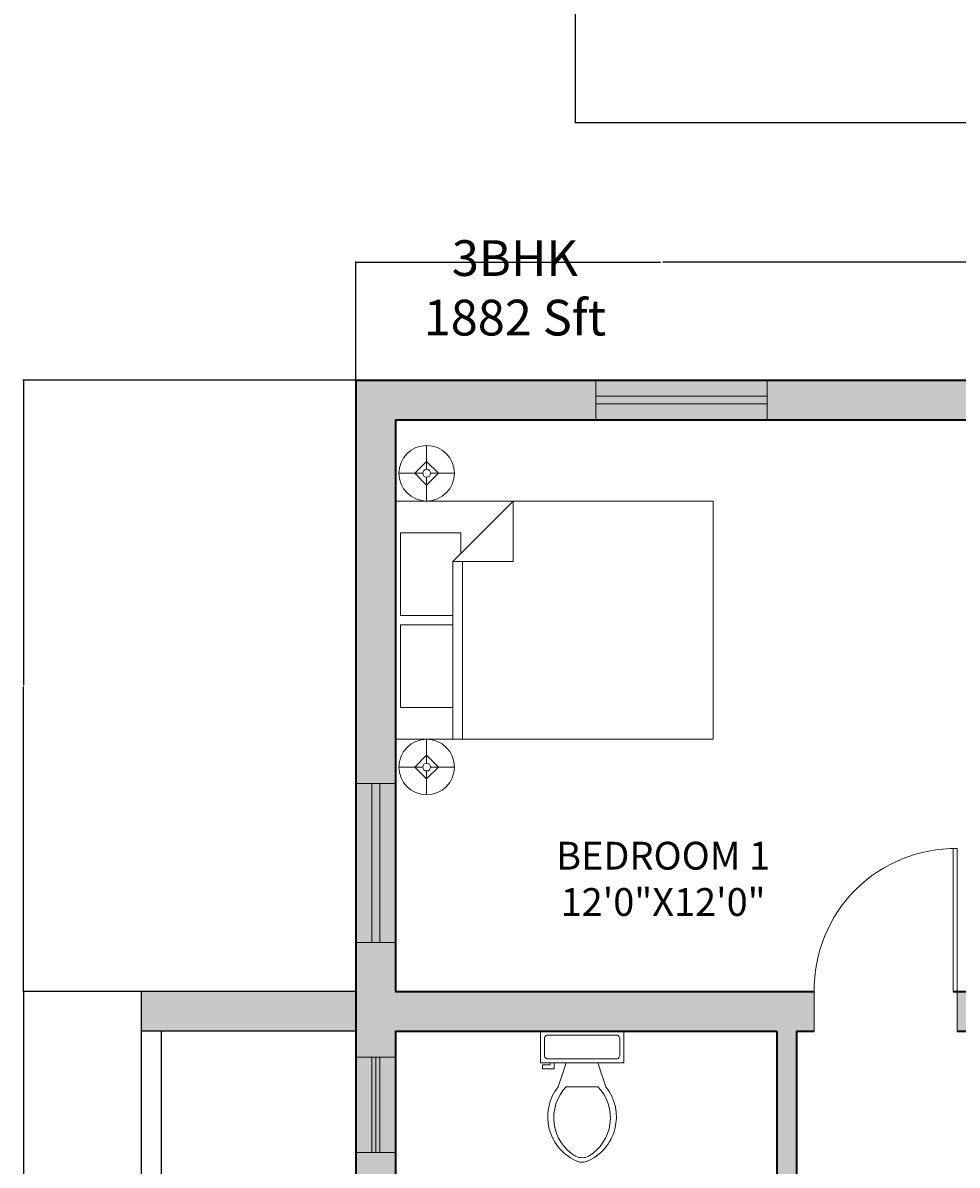
# Model space of a CAD drawing. Units: inches. Extents: x -382 to 250, y 518 to 1732.
# Tile 3 of 8: x -382 to -147, y 879 to 1167. Entities that reach past the tile are written whole.
import ezdxf

# ---------------------------------------------------------------- set-up
doc = ezdxf.new("R2010")
doc.units = ezdxf.units.IN
doc.header["$MEASUREMENT"] = 0
for name, color, linetype, lineweight in [('A-ANNO-DIMS', 2, 'Continuous', 18), ('A-ANNO-TEXT', 7, 'Continuous', 25), ('A-AREA-IDEN', 7, 'Continuous', 18), ('A-DOOR', 3, 'Continuous', 18), ('A-FLOR-EDGE', 7, 'Continuous', 25), ('A-FLOR-FIXT', 8, 'Continuous', 18), ('A-FURN', 8, 'Continuous', 18), ('A-GLAZ', 4, 'Continuous', 18), ('A-WALL', 7, 'Continuous', 35)]:
    doc.layers.add(name, color=color, linetype=linetype, lineweight=lineweight)
doc.layers.add('A-GLAZ-PATT', color=143, linetype='Continuous', lineweight=13, true_color=0x7aafdf)
doc.layers.add('A-WALL-PATT', color=251, linetype='Continuous', lineweight=13, true_color=0x636466)
doc.styles.get("Standard").update_dxf_attribs({"font": 'arial.ttf'})
doc.dimstyles.get("Standard").update_dxf_attribs({"dimtxt": 0.18, "dimasz": 0.18, "dimexe": 0.18, "dimexo": 0.0625, "dimgap": 0.09, "dimtad": 0, "dimtih": 1, "dimtoh": 1, "dimdec": 4, "dimzin": 0, "dimdsep": 46, "dimtxsty": 'Standard', "dimcen": 0.09, "dimadec": 0, "dimazin": 0, "dimtfac": 1, "dimtdec": 4, "dimtofl": 0, "dimtmove": 0, "dimatfit": 3, "dimfxl": 1, "dimtolj": 1, "dimtzin": 0, "dimarcsym": 0})

# ---------------------------------------------------------------- blocks, each defined once
blk = doc.blocks.new('Bed - Queen')
for p, q in [((0, -80.00003), (0, 0)), ((0, 0), (59.99999, 0)), ((59.99999, 0), (59.99999, -80.00003)), ((7.99999, -1.2), (28.79998, -1.2)), ((7.99999, -14.4), (7.99999, -1.2)), ((28.79998, -1.2), (28.79998, -14.4)), ((31.19999, -1.2), (51.99999, -1.2)), ((31.19999, -14.4), (31.19999, -1.2)), ((51.99999, -1.2), (51.99999, -16.4)), ((0, -14.4), (44.8, -14.4)), ((44.8, -16.8), (0, -16.8)), ((59.99999, -29.6), (44.8, -14.4)), ((44.8, -14.4), (44.8, -29.6)), ((51.99999, -16.4), (46.79936, -16.4)), ((44.8, -29.6), (59.99999, -29.6)), ((59.99999, -80.00003), (0, -80.00003))]:
    blk.add_line(p, q)
blk = doc.blocks.new('Toilet - top')
for p, q in [((9.5, -6), (9.5, -2)), ((-10, -8.5), (-8, -8.5)), ((-10, -9.5), (-10, -8.5)), ((-8, -8.5), (-8, -8)), ((-7, -8), (-7, -9.5)), ((-4, -8), (-6, -14)), ((4, -8), (6, -14)), ((-7, -9.5), (-10, -9.5)), ((4, -14), (-4, -14))]:
    blk.add_line(p, q)
blk.add_lwpolyline([(10.5, -8), (10.5, 0), (-10.5, 0), (-10.5, -8)], close=True)
for points in [[(-9.5, -2), (-9.5, -6)], [(8.5, -1), (-8.5, -1)], [(-8.5, -7), (8.5, -7)]]:
    blk.add_lwpolyline(points)
for centre, radius, start, end in [((-8.62, -1.88), 0.884, 81.8699, 188.1301), ((8.62, -1.88), 0.884, 351.8699, 98.1301), ((-8.62, -6.12), 0.884, 171.8699, 278.1301), ((8.62, -6.12), 0.884, 261.8699, 8.1301), ((3.52, -21.58), 12.17, 141.4691, 247.9714), ((4.2, -21.82), 11.33, 136.3677, 238.9468), ((-3.52, -21.58), 12.17, 292.0284, 38.5307), ((-4.2, -21.82), 11.33, 301.053, 43.6321), ((0, -27.88), 4, 245.7318, 294.2682), ((0, -29), 4, 254.8605, 285.1395)]:
    blk.add_arc(centre, radius, start, end)
blk = doc.blocks.new('Lamp - Table')
for p, q in [((0, 7), (0, 1)), ((0, 3), (-3, 0)), ((3, 0), (0, 3)), ((-1, 0), (-7, 0)), ((-3, 0), (0, -3)), ((0, -3), (3, 0)), ((1, 0), (7, 0)), ((0, -1), (0, -7))]:
    blk.add_line(p, q)
for radius in [7, 1]:
    blk.add_circle((0, 0), radius)
blk = doc.blocks.new('WIN-43_2IN')
for p, q in [((0, 10), (0, 0)), ((43.2, 10), (43.2, 0)), ((0, 6), (43.2, 6)), ((0, 4), (43.2, 4))]:
    blk.add_line(p, q)
blk = doc.blocks.new('WIN-40IN')
for p, q in [((10, 40), (0, 40)), ((4, 40), (4, 0)), ((6, 40), (6, 0)), ((10, 0), (0, 0))]:
    blk.add_line(p, q)
blk = doc.blocks.new('DOOR-SWING-36IN')
for p, q in [((-1, 0), (-1, 36)), ((0, 0), (0, 36))]:
    blk.add_line(p, q)
blk.add_arc((-0.5, 0.5), 35.5, 89.1931, 180.8069)
blk = doc.blocks.new('*D76')
at = {"layer": 'A-ANNO-DIMS', "color": 0, "lineweight": -2, "transparency": 16777216}
for p, q in [((-298.22, 1077.13), (-298.22, 1106.95)), ((-298.04, 1106.77), (-221.5, 1106.77)), ((-144.4, 1106.77), (-220.94, 1106.77)), ((-144.22, 1077.13), (-144.22, 1106.95))]:
    blk.add_line(p, q, dxfattribs=at)
at = {"layer": 'A-ANNO-DIMS', "color": 0, "transparency": 16777216}
for points in [[(-298.04, 1106.8), (-298.04, 1106.74), (-298.22, 1106.77)], [(-144.4, 1106.8), (-144.4, 1106.74), (-144.22, 1106.77)]]:
    blk.add_solid(points, dxfattribs=at)
at = {"layer": 'Defpoints', "color": 0, "transparency": 16777216}
for p in [(-144.22, 1106.77), (-298.22, 1077.07), (-144.22, 1077.07)]:
    blk.add_point(p, dxfattribs=at)
at = {"layer": 'A-ANNO-DIMS', "color": 0, "transparency": 16777216, "insert": (-221.22, 1106.77), "char_height": 0.18, "attachment_point": 5}
blk.add_mtext('\\A1;154', dxfattribs=at)
blk = doc.blocks.new('*D80')
at = {"layer": 'A-ANNO-DIMS', "color": 0, "lineweight": -2, "transparency": 16777216}
for p, q in [((-352.28, 923.07), (-382.1, 923.07)), ((-381.92, 922.89), (-381.92, 846.75)), ((-381.92, 770.25), (-381.92, 846.39)), ((-352.28, 770.07), (-382.1, 770.07))]:
    blk.add_line(p, q, dxfattribs=at)
at = {"layer": 'A-ANNO-DIMS', "color": 0, "transparency": 16777216}
for points in [[(-381.95, 922.89), (-381.89, 922.89), (-381.92, 923.07)], [(-381.95, 770.25), (-381.89, 770.25), (-381.92, 770.07)]]:
    blk.add_solid(points, dxfattribs=at)
at = {"layer": 'Defpoints', "color": 0, "transparency": 16777216}
for p in [(-381.92, 923.07), (-352.22, 923.07), (-352.22, 770.07)]:
    blk.add_point(p, dxfattribs=at)
at = {"layer": 'A-ANNO-DIMS', "color": 0, "transparency": 16777216, "insert": (-381.92, 846.57), "char_height": 0.18, "attachment_point": 5}
blk.add_mtext('\\A1;153', dxfattribs=at)
blk = doc.blocks.new('*D81')
at = {"layer": 'A-ANNO-DIMS', "color": 0, "lineweight": -2, "transparency": 16777216}
for p, q in [((-298.28, 1077.07), (-382.1, 1077.07)), ((-381.92, 1076.89), (-381.92, 1000.25)), ((-381.92, 923.25), (-381.92, 999.89)), ((-298.28, 923.07), (-382.1, 923.07))]:
    blk.add_line(p, q, dxfattribs=at)
at = {"layer": 'A-ANNO-DIMS', "color": 0, "transparency": 16777216}
for points in [[(-381.95, 1076.89), (-381.89, 1076.89), (-381.92, 1077.07)], [(-381.95, 923.25), (-381.89, 923.25), (-381.92, 923.07)]]:
    blk.add_solid(points, dxfattribs=at)
at = {"layer": 'Defpoints', "color": 0, "transparency": 16777216}
for p in [(-381.92, 1077.07), (-298.22, 1077.07), (-298.22, 923.07)]:
    blk.add_point(p, dxfattribs=at)
at = {"layer": 'A-ANNO-DIMS', "color": 0, "transparency": 16777216, "insert": (-381.92, 1000.07), "char_height": 0.18, "attachment_point": 5}
blk.add_mtext('\\A1;154', dxfattribs=at)
blk = doc.blocks.new('*D86')
at = {"layer": 'A-ANNO-DIMS', "color": 0, "lineweight": -2, "transparency": 16777216}
for p, q in [((-242.98, 1352.01), (-242.98, 1141.82)), ((219.78, 1197.01), (219.78, 1141.82)), ((-242.8, 1142), (-11.99, 1142)), ((219.6, 1142), (-11.2, 1142))]:
    blk.add_line(p, q, dxfattribs=at)
at = {"layer": 'A-ANNO-DIMS', "color": 0, "transparency": 16777216}
for points in [[(-242.8, 1142.03), (-242.8, 1141.97), (-242.98, 1142)], [(219.6, 1142.03), (219.6, 1141.97), (219.78, 1142)]]:
    blk.add_solid(points, dxfattribs=at)
at = {"layer": 'Defpoints', "color": 0, "transparency": 16777216}
for p in [(-242.98, 1352.07), (219.78, 1197.07), (219.78, 1142)]:
    blk.add_point(p, dxfattribs=at)
at = {"layer": 'A-ANNO-DIMS', "color": 0, "transparency": 16777216, "insert": (-11.6, 1142), "char_height": 0.18, "attachment_point": 5}
blk.add_mtext('\\A1;462.8', dxfattribs=at)

msp = doc.modelspace()

# ---------------------------------------------------------------- hatches: boundary and pattern name
at = {"layer": 'A-GLAZ-PATT'}
h = msp.add_hatch(color=256, dxfattribs=at)
h.dxf.hatch_style = 1
h.paths.add_polyline_path([(-194.615, 1077.0687), (-237.815, 1077.0687), (-237.815, 1073.0687), (-194.615, 1073.0687)])
h = msp.add_hatch(color=256, dxfattribs=at)
h.dxf.hatch_style = 1
h.paths.add_polyline_path([(-194.615, 1073.0687), (-237.815, 1073.0687), (-237.815, 1071.0687), (-194.615, 1071.0687)])
h = msp.add_hatch(color=256, dxfattribs=at)
h.dxf.hatch_style = 1
h.paths.add_polyline_path([(-194.615, 1071.0687), (-237.815, 1071.0687), (-237.815, 1067.0687), (-194.615, 1067.0687)])
h = msp.add_hatch(color=256, dxfattribs=at)
h.dxf.hatch_style = 1
h.paths.add_polyline_path([(-294.215, 975.4246), (-298.215, 975.4246), (-298.215, 935.4246), (-294.215, 935.4246)])
h = msp.add_hatch(color=256, dxfattribs=at)
h.dxf.hatch_style = 1
h.paths.add_polyline_path([(-292.215, 975.4246), (-294.215, 975.4246), (-294.215, 935.4246), (-292.215, 935.4246)])
h = msp.add_hatch(color=256, dxfattribs=at)
h.dxf.hatch_style = 1
h.paths.add_polyline_path([(-288.215, 975.4246), (-292.215, 975.4246), (-292.215, 935.4246), (-288.215, 935.4246)])
h = msp.add_hatch(color=256, dxfattribs=at)
h.dxf.hatch_style = 1
h.paths.add_polyline_path([(-294.215, 906.5114), (-298.215, 906.5114), (-298.215, 882.5114), (-294.215, 882.5114)])
h = msp.add_hatch(color=256, dxfattribs=at)
h.dxf.hatch_style = 1
h.paths.add_polyline_path([(-293.215, 906.5114), (-294.215, 906.5114), (-294.215, 882.5114), (-293.215, 882.5114)])
h = msp.add_hatch(color=256, dxfattribs=at)
h.dxf.hatch_style = 1
h.paths.add_polyline_path([(-292.215, 906.5114), (-293.215, 906.5114), (-293.215, 882.5114), (-292.215, 882.5114)])
h = msp.add_hatch(color=256, dxfattribs=at)
h.dxf.hatch_style = 1
h.paths.add_polyline_path([(-288.215, 906.5114), (-292.215, 906.5114), (-292.215, 882.5114), (-288.215, 882.5114)])
at = {"layer": 'A-WALL-PATT'}
h = msp.add_hatch(color=256, dxfattribs=at)
h.dxf.hatch_style = 1
h.paths.add_polyline_path([(-288.215, 1067.0687), (-237.815, 1067.0687), (-237.815, 1077.0687), (-298.215, 1077.0687), (-298.215, 975.4246), (-288.215, 975.4246)])
h = msp.add_hatch(color=256, dxfattribs=at)
h.dxf.hatch_style = 1
h.paths.add_polyline_path([(-121.6147, 1067.0687), (-121.6147, 1077.0687), (-194.615, 1077.0687), (-194.615, 1067.0687), (-144.215, 1067.0687), (-144.215, 1013.2912), (-134.215, 1013.2912), (-134.215, 1067.0687)])
h.paths.add_polyline_path([(-24.4384, 1067.0687), (-24.4384, 1077.0687), (-97.6147, 1077.0687), (-97.6147, 1067.0687), (-38.215, 1067.0687), (-38.215, 971.0687), (-134.215, 971.0687), (-134.215, 983.2912), (-144.215, 983.2912), (-144.215, 923.0687), (-146.7819, 923.0687), (-146.7819, 913.0687), (-134.215, 913.0687), (-134.215, 966.0687), (-38.215, 966.0687), (-38.215, 913.0687), (-28.215, 913.0687), (-17.6234, 913.0687), (-17.6234, 923.0687), (-28.215, 923.0687), (-28.215, 966.0687), (30.8449, 966.0687), (30.8449, 971.0687), (-28.215, 971.0687), (-28.215, 1067.0687)])
h.paths.add_polyline_path([(-0.4384, 1077.0687), (-0.4384, 1067.0687), (67.785, 1067.0687), (67.785, 971.0687), (60.8449, 971.0687), (60.8449, 966.0687), (67.785, 966.0687), (67.785, 923.0687), (18.3766, 923.0687), (18.3766, 913.0687), (209.785, 913.0687), (209.785, 895.1233), (219.785, 895.1233), (219.785, 913.0687), (219.785, 1077.0687), (165.385, 1077.0687), (165.385, 1067.0687), (209.785, 1067.0687), (209.785, 923.0687), (77.785, 923.0687), (77.785, 1067.0687), (122.185, 1067.0687), (122.185, 1077.0687)])
h = msp.add_hatch(color=256, dxfattribs=at)
h.dxf.hatch_style = 1
h.paths.add_polyline_path([(-298.215, 913.0687), (-298.215, 906.5114), (-292.215, 906.5114), (-292.215, 882.5114), (-298.215, 882.5114), (-298.215, 836.0687), (-298.215, 810.633), (-298.215, 770.0687), (-298.215, 760.1943), (-288.215, 760.1943), (-288.215, 770.0687), (-183.4355, 770.0687), (-183.4355, 780.0687), (-187.215, 780.0687), (-187.215, 836.0687), (-187.215, 913.0687), (-182.7819, 913.0687), (-182.7819, 923.0687), (-288.215, 923.0687), (-288.215, 935.4246), (-298.215, 935.4246)])
h.paths.add_polyline_path([(-288.215, 913.0687), (-192.215, 913.0687), (-192.215, 841.0687), (-231.9873, 841.0687), (-231.9873, 836.0687), (-192.215, 836.0687), (-192.215, 780.0687), (-288.215, 780.0687), (-288.215, 836.0687), (-257.0354, 836.0687), (-257.0354, 841.0687), (-288.215, 841.0687), (-288.215, 851.5748, -0.08437411), (-288.5907, 854.3175, -0.06817478), (-288.215, 856.5282)], flags=16)
h.paths.add_polyline_path([(-251.7597, 913.0687), (-230.7597, 913.0687), (-230.7597, 905.0687), (-237.2597, 905.0687), (-235.2598, 899.0688, -0.50132349), (-240.215, 880.2076, -0.13289091), (-242.3044, 880.2076, -0.50131678), (-247.2598, 899.0686), (-245.2597, 905.0687), (-248.2597, 905.0687), (-248.2597, 903.5687), (-251.2597, 903.5687), (-251.2597, 905.0687), (-251.7597, 905.0687)], flags=0)
h.paths.add_polyline_path([(-250.0097, 912.0687), (-232.7597, 912.0687, -0.41421356), (-231.7597, 911.3187), (-231.7597, 907.0687, -0.41421356), (-232.5097, 906.0687), (-249.7597, 906.0687, -0.41421356), (-250.7597, 906.8187), (-250.7597, 911.0687, -0.41421356)], flags=0)
h.paths.add_polyline_path([(-280.8452, 863.304, -0.08191995), (-276.0343, 863.9392, -0.08191995), (-271.2743, 862.9956, -0.09001579), (-267.4783, 860.7269, -0.10446928), (-264.8925, 857.2852, -0.11763426), (-264.1233, 853.5291, -0.11763426), (-265.1327, 849.8303, -0.10446928), (-267.9347, 846.5623, -0.09001579), (-271.8689, 844.5426, -0.08191995), (-276.6798, 843.9075, -0.08191995), (-281.4398, 844.851, -0.09001579), (-285.2358, 847.1198, -0.10446928), (-287.8216, 850.5614, -0.11763426), (-288.5907, 854.3175, -0.11763426), (-287.5814, 858.0163, -0.10446928), (-284.7794, 861.2843, -0.09001579)], flags=16)
h.paths.add_polyline_path([(-280.6571, 862.4148, -0.0811847), (-276.2281, 863.0748, -0.0811847), (-271.8193, 862.2903, -0.08956207), (-268.2852, 860.2819, -0.10467817), (-265.8411, 857.1765, -0.1186217), (-265.0707, 853.7642, -0.1186217), (-265.937, 850.3751, -0.10467817), (-268.4676, 847.3397, -0.08956207), (-272.0569, 845.4318, -0.0811847), (-276.486, 844.7718, -0.0811847), (-280.8947, 845.5563, -0.08956207), (-284.4288, 847.5647, -0.10467817), (-286.8729, 850.6701, -0.1186217), (-287.6433, 854.0824, -0.1186217), (-286.7771, 857.4715, -0.10467817), (-284.2464, 860.5069, -0.08956207)], flags=0)
h.paths.add_polyline_path([(-279.1993, 859.5164, -0.08143608), (-276.2895, 859.9601, -0.08143608), (-273.3904, 859.4514, -0.08971796), (-271.0622, 858.1333, -0.10460746), (-269.45, 856.0908, -0.11828257), (-268.9366, 853.8403, -0.11828257), (-269.5002, 851.6019, -0.10460746), (-271.1577, 849.596, -0.08971796), (-273.5148, 848.3302, -0.08143608), (-276.4245, 847.8865, -0.08143608), (-279.3236, 848.3952, -0.08971796), (-281.6518, 849.7133, -0.10460746), (-283.2641, 851.7558, -0.11828257), (-283.7775, 854.0063, -0.11828257), (-283.2139, 856.2447, -0.10460746), (-281.5563, 858.2507, -0.08971796)], flags=0)
h = msp.add_hatch(color=256, dxfattribs=at)
h.dxf.hatch_style = 1
h.paths.add_polyline_path([(-298.215, 923.0687), (-352.215, 923.0687), (-352.215, 913.0687), (-298.215, 913.0687)])

# ---------------------------------------------------------------- linework, layer by layer
at = {"layer": 'A-DOOR'}
for p, q in [((-182.7819, 923.0687), (-182.7819, 913.0687)), ((-146.7819, 923.0687), (-146.7819, 913.0687))]:
    msp.add_line(p, q, dxfattribs=at)
at = {"layer": 'A-FLOR-EDGE'}
for p, q in [((-298.215, 923.0687), (-352.215, 923.0687)), ((-352.215, 770.0687), (-352.215, 923.0687)), ((-298.215, 913.0687), (-352.215, 913.0687)), ((-347.215, 780.0687), (-347.215, 913.0687))]:
    msp.add_line(p, q, dxfattribs=at)
at = {"layer": 'A-GLAZ'}
for p, q in [((-288.215, 906.5114), (-298.215, 906.5114)), ((-294.215, 906.5114), (-294.215, 882.5114)), ((-293.215, 906.5114), (-293.215, 882.5114)), ((-292.215, 906.5114), (-292.215, 882.5114)), ((-288.215, 882.5114), (-298.215, 882.5114))]:
    msp.add_line(p, q, dxfattribs=at)
at = {"layer": 'A-WALL'}
for p, q in [((-298.215, 1077.0687), (-298.215, 913.0687)), ((-298.215, 1077.0687), (-134.215, 1077.0687)), ((-288.215, 1067.0687), (-288.215, 923.0687)), ((-288.215, 1067.0687), (-144.215, 1067.0687)), ((-288.215, 923.0687), (-182.7819, 923.0687)), ((-147.7819, 923.0687), (-144.215, 923.0687)), ((-298.215, 913.0687), (-298.215, 836.0687)), ((-288.215, 913.0687), (-192.215, 913.0687)), ((-288.215, 913.0687), (-288.215, 841.0687)), ((-192.215, 913.0687), (-192.215, 841.0687)), ((-187.215, 913.0687), (-187.215, 836.0687)), ((-187.215, 913.0687), (-182.7819, 913.0687)), ((-146.7819, 913.0687), (-134.215, 913.0687))]:
    msp.add_line(p, q, dxfattribs=at)

# ---------------------------------------------------------------- block references
at = {"layer": 'A-DOOR'}
msp.add_blockref('DOOR-SWING-36IN', (-146.7819, 923.0687), dxfattribs=at)
at = {"layer": 'A-FLOR-FIXT'}
msp.add_blockref('Toilet - top', (-241.2597, 913.0687), dxfattribs=at)
at = {"layer": 'A-FURN', "xscale": -1, "rotation": 90}
msp.add_blockref('Lamp - Table', (-280.4036, 1053.6072), dxfattribs=at)
at = {"layer": 'A-FURN', "rotation": 90}
for name, p in [('Bed - Queen', (-288.215, 986.6072)), ('Lamp - Table', (-280.4036, 979.6072))]:
    msp.add_blockref(name, p, dxfattribs=at)
at = {"layer": 'A-GLAZ'}
for name, p in [('WIN-43_2IN', (-237.815, 1067.069)), ('WIN-40IN', (-298.215, 935.4243))]:
    msp.add_blockref(name, p, dxfattribs=at)

# ---------------------------------------------------------------- texts
at = {"layer": 'A-ANNO-TEXT', "insert": (-321.76, 1112.3185), "char_height": 9, "attachment_point": 1}
msp.add_mtext_dynamic_manual_height_columns('\\pxqc;3BHK\\P1882 Sft', width=127.14497, gutter_width=1, heights=[0], dxfattribs=at)
at = {"layer": 'A-AREA-IDEN', "insert": (-260.6721, 960.7745), "char_height": 7, "attachment_point": 1}
msp.add_mtext_dynamic_manual_height_columns('\\pxqc;BEDROOM 1\\P12\'0"X12\'0"', width=79.656175, gutter_width=1, heights=[0], dxfattribs=at)

# ---------------------------------------------------------------- dimensions: what is measured, and where the dimension line sits
at = {"layer": 'A-ANNO-DIMS'}
for base, p1, p2, override, picture, middle in [((219.785, 1141.9977), (-242.9787, 1352.0687), (219.785, 1197.0687), {"dimdec": 1, "dimlfac": 1, "dimrnd": 0, "dimzin": 0, "dimdsep": 46, "dimlunit": 2}, '*D86', (-11.5969, 1141.9977)), ((-144.215, 1106.7687), (-298.215, 1077.0687), (-144.215, 1077.0687), {"dimdec": 0, "dimlfac": 1, "dimrnd": 0, "dimzin": 0, "dimdsep": 46, "dimlunit": 2}, '*D76', (-221.215, 1106.7687))]:
    dim = msp.add_linear_dim(base=base, p1=p1, p2=p2, dimstyle='Standard', override=override, dxfattribs=at)
    dim.commit()
    dim.dimension.update_dxf_attribs({"geometry": picture, "text_midpoint": middle})
for base, p1, p2, picture, middle in [((-381.915, 1077.0687), (-298.215, 923.0687), (-298.215, 1077.0687), '*D81', (-381.915, 1000.0687)), ((-381.915, 923.0687), (-352.215, 770.0687), (-352.215, 923.0687), '*D80', (-381.915, 846.5687))]:
    dim = msp.add_linear_dim(base=base, p1=p1, p2=p2, angle=90, dimstyle='Standard', override={"dimdec": 0, "dimlfac": 1, "dimrnd": 0, "dimzin": 0, "dimdsep": 46, "dimlunit": 2}, dxfattribs=at)
    dim.commit()
    dim.dimension.update_dxf_attribs({"geometry": picture, "text_midpoint": middle})

doc.saveas('drawing.dxf')
